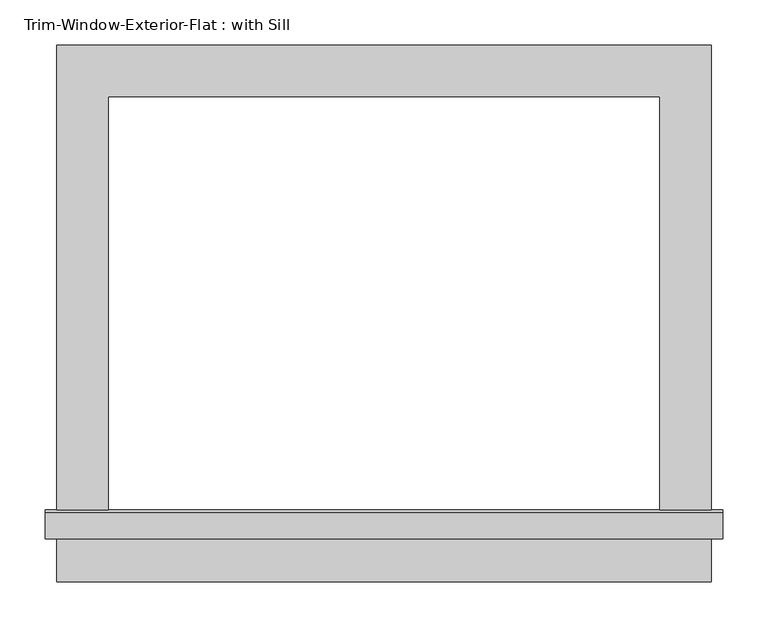
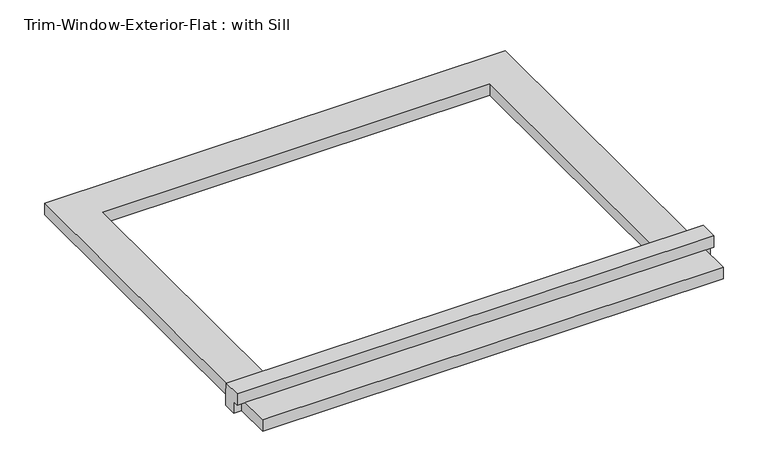
"""IFC4 building model written with IfcOpenShell, lengths in millimetres: proxy geometry, Trim-Window-Exterior-Flat : with Sill."""

from ifc_helpers import new_model, si_unit, frame, origin, origin_with_axes, place, context, project, spatial, polyline, outline, extrude, source, transform, mapped, element, save


def trim_window_exterior_flat_with_sill_f6d2a3b8(model_context):
    return source(origin(), model_context, "Body", "SweptSolid", [
        extrude(outline(polyline([(361.95, -479.3823709), (361.95, -536.5323709), (-361.95, -536.5323709), (-361.95, -479.3823709), (361.95, -479.3823709)])), origin_with_axes(), (0.0, 0.0, 1.0), 19.05),
        extrude(outline(polyline([(-488.95, 38.1), (-459.6580645, 38.1), (-457.2, 19.05), (-457.2, 0.0), (-479.3823709, 0.0), (-479.3823709, 19.05), (-488.95, 19.05), (-488.95, 38.1)])), frame((-374.65, 0.0, 0.0), z_axis=(1.0, 0.0, 0.0), x_axis=(0.0, 1.0, 0.0)), (0.0, 0.0, 1.0), 749.3),
        extrude(outline(polyline([(-361.95, 57.15), (361.95, 57.15), (361.95, -457.2), (304.8, -457.2), (304.8, 0.0), (-304.8, 0.0), (-304.8, -457.2), (-361.95, -457.2), (-361.95, 57.15)])), origin_with_axes(), (0.0, 0.0, 1.0), 19.05),
    ])


if __name__ == "__main__":
    model = new_model("IFC4")
    model_context = context("Model", 3, world=origin())
    ifc_project = project(units=[si_unit("LENGTHUNIT", "METRE", prefix="MILLI")], contexts=[model_context])
    site = spatial("IfcSite", under=ifc_project)
    building = spatial("IfcBuilding", under=site)
    placement = place(None, origin())
    trim_window_exterior_flat_with_sill_shape = trim_window_exterior_flat_with_sill_f6d2a3b8(model_context)
    element("IfcBuildingElementProxy", 1, Name="Trim-Window-Exterior-Flat : with Sill", ObjectType="Trim-Window-Exterior-Flat : with Sill", at=placement, inside=building, context=model_context, shape_type="MappedRepresentation", body=[
        mapped(trim_window_exterior_flat_with_sill_shape, transform((0.0, 0.0, 0.0), x_axis=(1.0, 0.0, 0.0), y_axis=(0.0, 1.0, 0.0), z_axis=(0.0, 0.0, 1.0))),
    ])
    save(model, "model.ifc")

# Revit data of these elements
# Type "Trim-Window-Exterior-Flat : with Sill"
#   Trim Width = 0' - 2 1/4"
#   Trim Thickness_Picture Frame = 0' - 1 1/4"
#   Trim Thickness_with Sill = 0' - 0 3/4"
#   Sill Thickness = 0' - 1 1/4"
#   Opening Width [instance default] = 2' - 0"
#   Opening Height [instance default] = 3' - 0"
#   Default Elevation = 4' - 0"
#   Sill = yes
#   Picture Frame = no
#   Trim Material [instance default] = none
# Element 1 (IfcBuildingElementProxy, "Trim-Window-Exterior-Flat : with Sill")
#   Opening Height = 1' - 6"
#   Trim Material = Clad - White
#   Materials on its faces: "Clad - White"
# Materials
#   "Clad - White": class "Wood", colour RGB 242 242 238, transparency 0, Cost = 0
